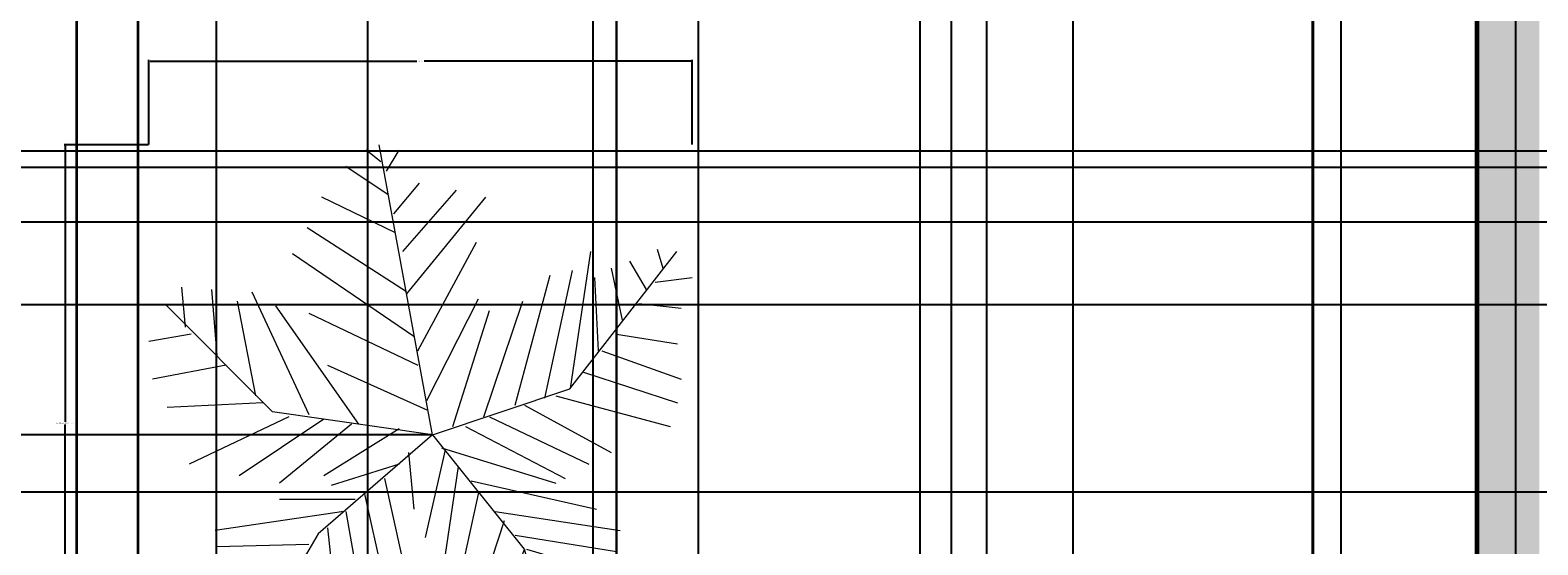
# Model space of a CAD drawing. Units: inches. Extents: x 818 to 1898, y 976 to 2364.
# Tile 8 of 96: x 986 to 1207, y 1592 to 1668. Entities that reach past the tile are written whole.
import ezdxf

# ---------------------------------------------------------------- set-up
doc = ezdxf.new("R2010")
doc.units = ezdxf.units.IN
doc.header["$LTSCALE"] = 5
doc.header["$MEASUREMENT"] = 0
for name, color, linetype, lineweight in [('A-ANNO-DIMS', 2, 'Continuous', 18), ('A-WALL', 7, 'Continuous', 40), ('C-PROP', 7, 'Continuous', 35), ('L-PLNT-BEDS', 94, 'Continuous', 18)]:
    doc.layers.add(name, color=color, linetype=linetype, lineweight=lineweight)
doc.layers.add('A-WALL-PATT', color=251, linetype='Continuous', lineweight=13, true_color=0x636466)
doc.layers.add('L-PLNT', color=116, linetype='Continuous', lineweight=13, true_color=0x136734)
doc.styles.get("Standard").update_dxf_attribs({"font": 'arial.ttf'})
doc.dimstyles.get("Standard").update_dxf_attribs({"dimtxt": 0.18, "dimasz": 0.18, "dimexe": 0.18, "dimexo": 0.0625, "dimgap": 0.09, "dimtad": 0, "dimtih": 1, "dimtoh": 1, "dimdec": 4, "dimzin": 0, "dimdsep": 46, "dimtxsty": 'Standard', "dimcen": 0.09, "dimadec": 0, "dimazin": 0, "dimtfac": 1, "dimtdec": 4, "dimtofl": 0, "dimtmove": 0, "dimatfit": 3, "dimfxl": 1, "dimtolj": 1, "dimtzin": 0, "dimarcsym": 0})

# ---------------------------------------------------------------- blocks, each defined once
blk = doc.blocks.new('PALM-BORDER')
for p, q in [((33.95, 78.95), (31.8, 80.68)), ((41.53, 39.05), (33.72, 81.45)), ((34.76, 77.57), (36.65, 80.68)), ((35.03, 74.11), (28.83, 78.26)), ((35.84, 71.35), (39.61, 75.84)), ((36.11, 68.59), (25.33, 73.77)), ((37.18, 65.82), (45, 74.8)), ((37.72, 59.6), (49.31, 73.77)), ((37.72, 59.95), (23.17, 69.28)), ((39.34, 51.31), (47.96, 67.2)), ((74.37, 66.17), (75.18, 63.4)), ((38.8, 53.39), (21.02, 65.48)), ((61.61, 45.75), (77.23, 65.83)), ((61.71, 45.79), (64.67, 65.82)), ((70.33, 64.44), (72.75, 60.3)), ((53.62, 43.37), (58.74, 62.37)), ((57.93, 44.41), (61.97, 63.06)), ((65.21, 62.02), (65.75, 51.31)), ((67.63, 63.4), (69.25, 55.81)), ((74.1, 61.33), (79.49, 62.02)), ((5.39, 54.77), (4.85, 60.64)), ((9.16, 60.3), (9.97, 50.62)), ((15.09, 59.95), (23.44, 41.99)), ((18.1, 42.4), (2.48, 58.02)), ((12.93, 58.57), (15.63, 44.75)), ((30.72, 40.61), (18.59, 57.88)), ((40.69, 44.06), (48.23, 58.91)), ((49.04, 41.64), (54.7, 58.57)), ((71.68, 58.22), (77.87, 57.53)), ((23.44, 56.84), (39.34, 49.24)), ((44.46, 40.26), (49.85, 57.19)), ((6.2, 53.73), (0, 52.7)), ((68.44, 53.73), (77.33, 52.35)), ((66.29, 51.31), (77.87, 47.17)), ((11.32, 49.24), (0.54, 47.17)), ((26.14, 49.24), (40.69, 42.68)), ((63.59, 48.21), (77.33, 43.71)), ((41.53, 39.05), (61.61, 45.75)), ((59.55, 44.75), (76.26, 40.26)), ((16.71, 43.71), (2.69, 43.02)), ((41.53, 39.05), (18.1, 42.4)), ((54.97, 43.37), (67.63, 36.46)), ((20.48, 41.64), (5.93, 34.73)), ((25.6, 41.3), (13.2, 33.01)), ((29.64, 40.61), (19.13, 31.97)), ((36.65, 39.91), (25.6, 33.01)), ((46.35, 40.26), (60.9, 32.66)), ((49.85, 41.64), (64.4, 34.73)), ((41.53, 39.05), (24.79, 24.55)), ((41.53, 39.05), (54.92, 22.32)), ((37.99, 36.46), (38.8, 28.17)), ((43.38, 36.81), (40.42, 24.02)), ((42.84, 37.15), (59.55, 31.97)), ((36.65, 34.73), (26.68, 31.62)), ((45.27, 34.39), (43.11, 19.88)), ((34.49, 32.66), (36.92, 21.61)), ((47.15, 32.32), (65.48, 28.17)), ((30.18, 29.55), (19.13, 29.55)), ((31.53, 30.59), (35.03, 14.7)), ((48.23, 30.59), (44.19, 12.28)), ((28.56, 27.82), (9.7, 25.06)), ((28.83, 27.82), (32.07, 9.17)), ((50.66, 27.82), (68.98, 25.06)), ((24.79, 24.55), (13.63, 5.58)), ((26.14, 25.41), (28.29, 6.06)), ((52, 26.44), (46.35, 9.17)), ((53.62, 24.37), (68.44, 21.95)), ((23.44, 22.99), (9.97, 22.64)), ((54.97, 22.3), (47.69, 5.02)), ((54.92, 22.32), (61.61, 0)), ((55.24, 22.3), (71.68, 17.46)), ((21.56, 19.53), (11.59, 19.88)), ((22.9, 21.26), (24.52, 5.37)), ((55.78, 20.22), (70.33, 14.35)), ((20.48, 17.46), (9.7, 15.73)), ((19.94, 16.08), (20.75, 6.41)), ((56.59, 16.42), (53.35, 5.72)), ((18.59, 13.66), (9.97, 12.62)), ((57.39, 14.7), (70.6, 8.83)), ((17.24, 11.59), (17.78, 6.06)), ((15.9, 9.52), (11.05, 7.44)), ((58.47, 10.9), (56.05, 2.95)), ((58.47, 10.55), (67.09, 5.72)), ((59.82, 6.75), (64.4, 3.64)), ((59.82, 5.02), (58.74, 1.22)), ((61.44, 1.92), (62.51, 1.22))]:
    blk.add_line(p, q)
blk = doc.blocks.new('*D26')
at = {"layer": 'A-ANNO-DIMS', "color": 0, "lineweight": -2, "ltscale": 5, "transparency": 16777216}
for p, q in [((1003.26, 1650.91), (990.92, 1650.91)), ((991.1, 1650.73), (991.1, 1610.37)), ((991.1, 1569.64), (991.1, 1610)), ((1003.26, 1569.46), (990.92, 1569.46))]:
    blk.add_line(p, q, dxfattribs=at)
at = {"layer": 'A-ANNO-DIMS', "color": 0, "ltscale": 5, "transparency": 16777216}
for points in [[(991.07, 1650.73), (991.13, 1650.73), (991.1, 1650.91)], [(991.07, 1569.64), (991.13, 1569.64), (991.1, 1569.46)]]:
    blk.add_solid(points, dxfattribs=at)
at = {"layer": 'Defpoints', "color": 0, "ltscale": 5, "transparency": 16777216}
for p in [(991.1, 1650.91), (1003.32, 1650.91), (1003.32, 1569.46)]:
    blk.add_point(p, dxfattribs=at)
at = {"layer": 'A-ANNO-DIMS', "color": 0, "ltscale": 5, "transparency": 16777216, "insert": (991.1, 1610.19), "char_height": 0.18, "attachment_point": 5}
blk.add_mtext('\\A1;BORDER PALM 81 TYP.', dxfattribs=at)
blk = doc.blocks.new('*D27')
at = {"layer": 'A-ANNO-DIMS', "color": 0, "lineweight": -2, "ltscale": 5, "transparency": 16777216}
for p, q in [((1003.32, 1650.97), (1003.32, 1663.31)), ((1003.5, 1663.13), (1042.54, 1663.13)), ((1082.63, 1663.13), (1043.59, 1663.13)), ((1082.81, 1650.97), (1082.81, 1663.31))]:
    blk.add_line(p, q, dxfattribs=at)
at = {"layer": 'A-ANNO-DIMS', "color": 0, "ltscale": 5, "transparency": 16777216}
for points in [[(1003.5, 1663.16), (1003.5, 1663.1), (1003.32, 1663.13)], [(1082.63, 1663.16), (1082.63, 1663.1), (1082.81, 1663.13)]]:
    blk.add_solid(points, dxfattribs=at)
at = {"layer": 'Defpoints', "color": 0, "ltscale": 5, "transparency": 16777216}
for p in [(1082.81, 1663.13), (1003.32, 1650.91), (1082.81, 1650.91)]:
    blk.add_point(p, dxfattribs=at)
at = {"layer": 'A-ANNO-DIMS', "color": 0, "ltscale": 5, "transparency": 16777216, "insert": (1043.06, 1663.13), "char_height": 0.18, "attachment_point": 5}
blk.add_mtext('\\A1;79 TYP.', dxfattribs=at)
blk = doc.blocks.new('*D59')
at = {"layer": 'A-ANNO-DIMS', "color": 0, "lineweight": -2, "ltscale": 5, "transparency": 16777216}
for p, q in [((1251.64, 2300.39), (818.03, 2300.39)), ((818.21, 2300.21), (818.21, 1669.95)), ((818.21, 1039.32), (818.21, 1669.59)), ((896.05, 1039.14), (818.03, 1039.14))]:
    blk.add_line(p, q, dxfattribs=at)
at = {"layer": 'A-ANNO-DIMS', "color": 0, "ltscale": 5, "transparency": 16777216}
for points in [[(818.18, 2300.21), (818.24, 2300.21), (818.21, 2300.39)], [(818.18, 1039.32), (818.24, 1039.32), (818.21, 1039.14)]]:
    blk.add_solid(points, dxfattribs=at)
at = {"layer": 'Defpoints', "color": 0, "ltscale": 5, "transparency": 16777216}
for p in [(818.21, 2300.39), (1251.71, 2300.39), (896.11, 1039.14)]:
    blk.add_point(p, dxfattribs=at)
at = {"layer": 'A-ANNO-DIMS', "color": 0, "ltscale": 5, "transparency": 16777216, "insert": (818.21, 1669.77), "char_height": 0.18, "attachment_point": 5}
blk.add_mtext('\\A1;1261.2', dxfattribs=at)
blk = doc.blocks.new('*D60')
at = {"layer": 'A-ANNO-DIMS', "color": 0, "lineweight": -2, "ltscale": 5, "transparency": 16777216}
for p, q in [((992.66, 2294.22), (818.03, 2294.22)), ((818.21, 2294.04), (818.21, 1748.77)), ((818.21, 1203.14), (818.21, 1748.41)), ((992.66, 1202.96), (818.03, 1202.96))]:
    blk.add_line(p, q, dxfattribs=at)
at = {"layer": 'A-ANNO-DIMS', "color": 0, "ltscale": 5, "transparency": 16777216}
for points in [[(818.18, 2294.04), (818.24, 2294.04), (818.21, 2294.22)], [(818.18, 1203.14), (818.24, 1203.14), (818.21, 1202.96)]]:
    blk.add_solid(points, dxfattribs=at)
at = {"layer": 'Defpoints', "color": 0, "ltscale": 5, "transparency": 16777216}
for p in [(818.21, 2294.22), (992.73, 2294.22), (992.73, 1202.96)]:
    blk.add_point(p, dxfattribs=at)
at = {"layer": 'A-ANNO-DIMS', "color": 0, "ltscale": 5, "transparency": 16777216, "insert": (818.21, 1748.59), "char_height": 0.18, "attachment_point": 5}
blk.add_mtext('\\A1;1091.3', dxfattribs=at)
blk = doc.blocks.new('*D61')
at = {"layer": 'A-ANNO-DIMS', "color": 0, "lineweight": -2, "ltscale": 5, "transparency": 16777216}
for p, q in [((1071.73, 1203.03), (1071.73, 2363.87)), ((1071.91, 2363.69), (1250.94, 2363.69)), ((1430.55, 2363.69), (1251.51, 2363.69)), ((1430.73, 1203.03), (1430.73, 2363.87))]:
    blk.add_line(p, q, dxfattribs=at)
at = {"layer": 'A-ANNO-DIMS', "color": 0, "ltscale": 5, "transparency": 16777216}
for points in [[(1071.91, 2363.72), (1071.91, 2363.66), (1071.73, 2363.69)], [(1430.55, 2363.72), (1430.55, 2363.66), (1430.73, 2363.69)]]:
    blk.add_solid(points, dxfattribs=at)
at = {"layer": 'Defpoints', "color": 0, "ltscale": 5, "transparency": 16777216}
for p in [(1430.73, 2363.69), (1071.73, 1202.96), (1430.73, 1202.96)]:
    blk.add_point(p, dxfattribs=at)
at = {"layer": 'A-ANNO-DIMS', "color": 0, "ltscale": 5, "transparency": 16777216, "insert": (1251.23, 2363.69), "char_height": 0.18, "attachment_point": 5}
blk.add_mtext('\\A1;359', dxfattribs=at)
blk = doc.blocks.new('*D64')
at = {"layer": 'A-ANNO-DIMS', "color": 0, "lineweight": -2, "ltscale": 5, "transparency": 16777216}
for p, q in [((1197.73, 1501.14), (1197.73, 2363.87)), ((1197.91, 2363.69), (1313.93, 2363.69)), ((1430.55, 2363.69), (1314.52, 2363.69)), ((1430.73, 1501.14), (1430.73, 2363.87))]:
    blk.add_line(p, q, dxfattribs=at)
at = {"layer": 'A-ANNO-DIMS', "color": 0, "ltscale": 5, "transparency": 16777216}
for points in [[(1197.91, 2363.72), (1197.91, 2363.66), (1197.73, 2363.69)], [(1430.55, 2363.72), (1430.55, 2363.66), (1430.73, 2363.69)]]:
    blk.add_solid(points, dxfattribs=at)
at = {"layer": 'Defpoints', "color": 0, "ltscale": 5, "transparency": 16777216}
for p in [(1430.73, 2363.69), (1197.73, 1501.08), (1430.73, 1501.08)]:
    blk.add_point(p, dxfattribs=at)
at = {"layer": 'A-ANNO-DIMS', "color": 0, "ltscale": 5, "transparency": 16777216, "insert": (1314.23, 2363.69), "char_height": 0.18, "attachment_point": 5}
blk.add_mtext('\\A1;233', dxfattribs=at)
blk = doc.blocks.new('*D79')
at = {"layer": 'A-ANNO-DIMS', "color": 0, "lineweight": -2, "ltscale": 5, "transparency": 16777216}
for p, q in [((992.73, 1203.03), (992.73, 2363.87)), ((992.91, 2363.69), (1032.01, 2363.69)), ((1071.55, 2363.69), (1032.44, 2363.69)), ((1071.73, 1203.03), (1071.73, 2363.87))]:
    blk.add_line(p, q, dxfattribs=at)
at = {"layer": 'A-ANNO-DIMS', "color": 0, "ltscale": 5, "transparency": 16777216}
for points in [[(992.91, 2363.72), (992.91, 2363.66), (992.73, 2363.69)], [(1071.55, 2363.72), (1071.55, 2363.66), (1071.73, 2363.69)]]:
    blk.add_solid(points, dxfattribs=at)
at = {"layer": 'Defpoints', "color": 0, "ltscale": 5, "transparency": 16777216}
for p in [(1071.73, 2363.69), (992.73, 1202.96), (1071.73, 1202.96)]:
    blk.add_point(p, dxfattribs=at)
at = {"layer": 'A-ANNO-DIMS', "color": 0, "ltscale": 5, "transparency": 16777216, "insert": (1032.23, 2363.69), "char_height": 0.18, "attachment_point": 5}
blk.add_mtext('\\A1;79', dxfattribs=at)
blk = doc.blocks.new('*D82')
at = {"layer": 'A-ANNO-DIMS', "color": 0, "lineweight": -2, "ltscale": 5, "transparency": 16777216}
for p, q in [((1083.73, 1501.14), (1083.73, 2363.87)), ((1083.91, 2363.69), (1140.45, 2363.69)), ((1197.55, 2363.69), (1141.01, 2363.69)), ((1197.73, 1501.14), (1197.73, 2363.87))]:
    blk.add_line(p, q, dxfattribs=at)
at = {"layer": 'A-ANNO-DIMS', "color": 0, "ltscale": 5, "transparency": 16777216}
for points in [[(1083.91, 2363.72), (1083.91, 2363.66), (1083.73, 2363.69)], [(1197.55, 2363.72), (1197.55, 2363.66), (1197.73, 2363.69)]]:
    blk.add_solid(points, dxfattribs=at)
at = {"layer": 'Defpoints', "color": 0, "ltscale": 5, "transparency": 16777216}
for p in [(1197.73, 2363.69), (1083.73, 1501.08), (1197.73, 1501.08)]:
    blk.add_point(p, dxfattribs=at)
at = {"layer": 'A-ANNO-DIMS', "color": 0, "ltscale": 5, "transparency": 16777216, "insert": (1140.73, 2363.69), "char_height": 0.18, "attachment_point": 5}
blk.add_mtext('\\A1;114', dxfattribs=at)
blk = doc.blocks.new('*D84')
at = {"layer": 'A-ANNO-DIMS', "color": 0, "lineweight": -2, "ltscale": 5, "transparency": 16777216}
for p, q in [((1197.66, 1700.08), (818.03, 1700.08)), ((818.21, 1699.9), (818.21, 1600.76)), ((818.21, 1501.26), (818.21, 1600.4)), ((1197.66, 1501.08), (818.03, 1501.08))]:
    blk.add_line(p, q, dxfattribs=at)
at = {"layer": 'A-ANNO-DIMS', "color": 0, "ltscale": 5, "transparency": 16777216}
for points in [[(818.18, 1699.9), (818.24, 1699.9), (818.21, 1700.08)], [(818.18, 1501.26), (818.24, 1501.26), (818.21, 1501.08)]]:
    blk.add_solid(points, dxfattribs=at)
at = {"layer": 'Defpoints', "color": 0, "ltscale": 5, "transparency": 16777216}
for p in [(818.21, 1700.08), (1197.73, 1700.08), (1197.73, 1501.08)]:
    blk.add_point(p, dxfattribs=at)
at = {"layer": 'A-ANNO-DIMS', "color": 0, "ltscale": 5, "transparency": 16777216, "insert": (818.21, 1600.58), "char_height": 0.18, "attachment_point": 5}
blk.add_mtext('\\A1;199', dxfattribs=at)
blk = doc.blocks.new('*D91')
at = {"layer": 'A-ANNO-DIMS', "color": 0, "lineweight": -2, "ltscale": 5, "transparency": 16777216}
for p, q in [((959.17, 1071.12), (959.17, 2363.87)), ((959.35, 2363.69), (985.8, 2363.69)), ((1013.04, 2363.69), (986.59, 2363.69)), ((1013.22, 1071.12), (1013.22, 2363.87))]:
    blk.add_line(p, q, dxfattribs=at)
at = {"layer": 'A-ANNO-DIMS', "color": 0, "ltscale": 5, "transparency": 16777216}
for points in [[(959.35, 2363.72), (959.35, 2363.66), (959.17, 2363.69)], [(1013.04, 2363.72), (1013.04, 2363.66), (1013.22, 2363.69)]]:
    blk.add_solid(points, dxfattribs=at)
at = {"layer": 'Defpoints', "color": 0, "ltscale": 5, "transparency": 16777216}
for p in [(1013.22, 2363.69), (959.17, 1071.06), (1013.22, 1071.06)]:
    blk.add_point(p, dxfattribs=at)
at = {"layer": 'A-ANNO-DIMS', "color": 0, "ltscale": 5, "transparency": 16777216, "insert": (986.2, 2363.69), "char_height": 0.18, "attachment_point": 5}
blk.add_mtext('\\A1;54.04', dxfattribs=at)
blk = doc.blocks.new('*D92')
at = {"layer": 'A-ANNO-DIMS', "color": 0, "lineweight": -2, "ltscale": 5, "transparency": 16777216}
for p, q in [((1013.22, 1071.12), (1013.22, 2363.87)), ((1013.4, 2363.69), (1040.38, 2363.69)), ((1068.16, 2363.69), (1041.17, 2363.69)), ((1068.34, 1071.12), (1068.34, 2363.87))]:
    blk.add_line(p, q, dxfattribs=at)
at = {"layer": 'A-ANNO-DIMS', "color": 0, "ltscale": 5, "transparency": 16777216}
for points in [[(1013.4, 2363.72), (1013.4, 2363.66), (1013.22, 2363.69)], [(1068.16, 2363.72), (1068.16, 2363.66), (1068.34, 2363.69)]]:
    blk.add_solid(points, dxfattribs=at)
at = {"layer": 'Defpoints', "color": 0, "ltscale": 5, "transparency": 16777216}
for p in [(1068.34, 2363.69), (1013.22, 1071.06), (1068.34, 1071.06)]:
    blk.add_point(p, dxfattribs=at)
at = {"layer": 'A-ANNO-DIMS', "color": 0, "ltscale": 5, "transparency": 16777216, "insert": (1040.78, 2363.69), "char_height": 0.18, "attachment_point": 5}
blk.add_mtext('\\A1;55.12', dxfattribs=at)
blk = doc.blocks.new('*D93')
at = {"layer": 'A-ANNO-DIMS', "color": 0, "lineweight": -2, "ltscale": 5, "transparency": 16777216}
for p, q in [((1068.34, 1071.12), (1068.34, 2363.87)), ((1068.52, 2363.69), (1094.16, 2363.69)), ((1120.58, 2363.69), (1094.94, 2363.69)), ((1120.76, 1071.12), (1120.76, 2363.87))]:
    blk.add_line(p, q, dxfattribs=at)
at = {"layer": 'A-ANNO-DIMS', "color": 0, "ltscale": 5, "transparency": 16777216}
for points in [[(1068.52, 2363.72), (1068.52, 2363.66), (1068.34, 2363.69)], [(1120.58, 2363.72), (1120.58, 2363.66), (1120.76, 2363.69)]]:
    blk.add_solid(points, dxfattribs=at)
at = {"layer": 'Defpoints', "color": 0, "ltscale": 5, "transparency": 16777216}
for p in [(1120.76, 2363.69), (1068.34, 1071.06), (1120.76, 1071.06)]:
    blk.add_point(p, dxfattribs=at)
at = {"layer": 'A-ANNO-DIMS', "color": 0, "ltscale": 5, "transparency": 16777216, "insert": (1094.55, 2363.69), "char_height": 0.18, "attachment_point": 5}
blk.add_mtext('\\A1;52.42', dxfattribs=at)
blk = doc.blocks.new('*D94')
at = {"layer": 'A-ANNO-DIMS', "color": 0, "lineweight": -2, "ltscale": 5, "transparency": 16777216}
for p, q in [((1120.76, 1071.12), (1120.76, 2363.87)), ((1120.94, 2363.69), (1146.76, 2363.69)), ((1173.36, 2363.69), (1147.55, 2363.69)), ((1173.54, 1071.12), (1173.54, 2363.87))]:
    blk.add_line(p, q, dxfattribs=at)
at = {"layer": 'A-ANNO-DIMS', "color": 0, "ltscale": 5, "transparency": 16777216}
for points in [[(1120.94, 2363.72), (1120.94, 2363.66), (1120.76, 2363.69)], [(1173.36, 2363.72), (1173.36, 2363.66), (1173.54, 2363.69)]]:
    blk.add_solid(points, dxfattribs=at)
at = {"layer": 'Defpoints', "color": 0, "ltscale": 5, "transparency": 16777216}
for p in [(1173.54, 2363.69), (1120.76, 1071.06), (1173.54, 1071.06)]:
    blk.add_point(p, dxfattribs=at)
at = {"layer": 'A-ANNO-DIMS', "color": 0, "ltscale": 5, "transparency": 16777216, "insert": (1147.15, 2363.69), "char_height": 0.18, "attachment_point": 5}
blk.add_mtext('\\A1;52.78', dxfattribs=at)
blk = doc.blocks.new('*D95')
at = {"layer": 'A-ANNO-DIMS', "color": 0, "lineweight": -2, "ltscale": 5, "transparency": 16777216}
for p, q in [((1173.54, 1071.12), (1173.54, 2363.87)), ((1173.72, 2363.69), (1201.29, 2363.69)), ((1229.47, 2363.69), (1201.9, 2363.69)), ((1229.65, 1071.12), (1229.65, 2363.87))]:
    blk.add_line(p, q, dxfattribs=at)
at = {"layer": 'A-ANNO-DIMS', "color": 0, "ltscale": 5, "transparency": 16777216}
for points in [[(1173.72, 2363.72), (1173.72, 2363.66), (1173.54, 2363.69)], [(1229.47, 2363.72), (1229.47, 2363.66), (1229.65, 2363.69)]]:
    blk.add_solid(points, dxfattribs=at)
at = {"layer": 'Defpoints', "color": 0, "ltscale": 5, "transparency": 16777216}
for p in [(1229.65, 2363.69), (1173.54, 1071.06), (1229.65, 1071.06)]:
    blk.add_point(p, dxfattribs=at)
at = {"layer": 'A-ANNO-DIMS', "color": 0, "ltscale": 5, "transparency": 16777216, "insert": (1201.59, 2363.69), "char_height": 0.18, "attachment_point": 5}
blk.add_mtext('\\A1;56.1', dxfattribs=at)
blk = doc.blocks.new('*D109')
at = {"layer": 'A-ANNO-DIMS', "color": 0, "lineweight": -2, "ltscale": 5, "transparency": 16777216}
for p, q in [((1125.92, 1410.12), (1125.92, 2363.87)), ((1126.1, 2363.69), (1164.25, 2363.69)), ((1203.15, 2363.69), (1165, 2363.69)), ((1203.33, 1409.91), (1203.33, 2363.87))]:
    blk.add_line(p, q, dxfattribs=at)
at = {"layer": 'A-ANNO-DIMS', "color": 0, "ltscale": 5, "transparency": 16777216}
for points in [[(1126.1, 2363.72), (1126.1, 2363.66), (1125.92, 2363.69)], [(1203.15, 2363.72), (1203.15, 2363.66), (1203.33, 2363.69)]]:
    blk.add_solid(points, dxfattribs=at)
at = {"layer": 'Defpoints', "color": 0, "ltscale": 5, "transparency": 16777216}
for p in [(1203.33, 2363.69), (1125.92, 1410.05), (1203.33, 1409.85)]:
    blk.add_point(p, dxfattribs=at)
at = {"layer": 'A-ANNO-DIMS', "color": 0, "ltscale": 5, "transparency": 16777216, "insert": (1164.62, 2363.69), "char_height": 0.18, "attachment_point": 5}
blk.add_mtext('\\A1;77.41', dxfattribs=at)
blk = doc.blocks.new('*D118')
at = {"layer": 'A-ANNO-DIMS', "color": 0, "lineweight": -2, "ltscale": 5, "transparency": 16777216}
for p, q in [((1766.29, 1627.51), (818.03, 1627.51)), ((818.21, 1627.33), (818.21, 1586.53)), ((818.21, 1545.36), (818.21, 1586.16)), ((1766.29, 1545.18), (818.03, 1545.18))]:
    blk.add_line(p, q, dxfattribs=at)
at = {"layer": 'A-ANNO-DIMS', "color": 0, "ltscale": 5, "transparency": 16777216}
for points in [[(818.18, 1627.33), (818.24, 1627.33), (818.21, 1627.51)], [(818.18, 1545.36), (818.24, 1545.36), (818.21, 1545.18)]]:
    blk.add_solid(points, dxfattribs=at)
at = {"layer": 'Defpoints', "color": 0, "ltscale": 5, "transparency": 16777216}
for p in [(818.21, 1627.51), (1766.35, 1627.51), (1766.35, 1545.18)]:
    blk.add_point(p, dxfattribs=at)
at = {"layer": 'A-ANNO-DIMS', "color": 0, "ltscale": 5, "transparency": 16777216, "insert": (818.21, 1586.34), "char_height": 0.18, "attachment_point": 5}
blk.add_mtext('\\A1;82.32', dxfattribs=at)
blk = doc.blocks.new('*D119')
at = {"layer": 'A-ANNO-DIMS', "color": 0, "lineweight": -2, "ltscale": 5, "transparency": 16777216}
for p, q in [((1766.29, 1716.99), (818.03, 1716.99)), ((818.21, 1716.81), (818.21, 1672.43)), ((818.21, 1627.69), (818.21, 1672.06)), ((1766.29, 1627.51), (818.03, 1627.51))]:
    blk.add_line(p, q, dxfattribs=at)
at = {"layer": 'A-ANNO-DIMS', "color": 0, "ltscale": 5, "transparency": 16777216}
for points in [[(818.18, 1716.81), (818.24, 1716.81), (818.21, 1716.99)], [(818.18, 1627.69), (818.24, 1627.69), (818.21, 1627.51)]]:
    blk.add_solid(points, dxfattribs=at)
at = {"layer": 'Defpoints', "color": 0, "ltscale": 5, "transparency": 16777216}
for p in [(818.21, 1716.99), (1766.35, 1716.99), (1766.35, 1627.51)]:
    blk.add_point(p, dxfattribs=at)
at = {"layer": 'A-ANNO-DIMS', "color": 0, "ltscale": 5, "transparency": 16777216, "insert": (818.21, 1672.25), "char_height": 0.18, "attachment_point": 5}
blk.add_mtext('\\A1;89.48', dxfattribs=at)
blk = doc.blocks.new('*D122')
at = {"layer": 'A-ANNO-DIMS', "color": 0, "lineweight": -2, "ltscale": 5, "transparency": 16777216}
for p, q in [((1138.5, 1794.37), (1138.5, 975.66)), ((1071.73, 1688.02), (1071.73, 975.66)), ((1071.91, 975.84), (1104.72, 975.84)), ((1138.32, 975.84), (1105.51, 975.84))]:
    blk.add_line(p, q, dxfattribs=at)
at = {"layer": 'A-ANNO-DIMS', "color": 0, "ltscale": 5, "transparency": 16777216}
for points in [[(1071.91, 975.87), (1071.91, 975.81), (1071.73, 975.84)], [(1138.32, 975.87), (1138.32, 975.81), (1138.5, 975.84)]]:
    blk.add_solid(points, dxfattribs=at)
at = {"layer": 'Defpoints', "color": 0, "ltscale": 5, "transparency": 16777216}
for p in [(1138.5, 1794.43), (1071.73, 1688.08), (1138.5, 975.84)]:
    blk.add_point(p, dxfattribs=at)
at = {"layer": 'A-ANNO-DIMS', "color": 0, "ltscale": 5, "transparency": 16777216, "insert": (1105.11, 975.84), "char_height": 0.18, "attachment_point": 5}
blk.add_mtext('\\A1;66.78', dxfattribs=at)
blk = doc.blocks.new('*D126')
at = {"layer": 'A-ANNO-DIMS', "color": 0, "lineweight": -2, "ltscale": 5, "transparency": 16777216}
for p, q in [((1035.38, 1252.09), (1035.38, 2363.87)), ((1035.56, 2363.69), (1075.41, 2363.69)), ((1116.01, 2363.69), (1076.16, 2363.69)), ((1116.19, 1236.03), (1116.19, 2363.87))]:
    blk.add_line(p, q, dxfattribs=at)
at = {"layer": 'A-ANNO-DIMS', "color": 0, "ltscale": 5, "transparency": 16777216}
for points in [[(1035.56, 2363.72), (1035.56, 2363.66), (1035.38, 2363.69)], [(1116.01, 2363.72), (1116.01, 2363.66), (1116.19, 2363.69)]]:
    blk.add_solid(points, dxfattribs=at)
at = {"layer": 'Defpoints', "color": 0, "ltscale": 5, "transparency": 16777216}
for p in [(1035.38, 2363.69), (1035.38, 1252.02), (1116.19, 1235.96)]:
    blk.add_point(p, dxfattribs=at)
at = {"layer": 'A-ANNO-DIMS', "color": 0, "ltscale": 5, "transparency": 16777216, "insert": (1075.78, 2363.69), "char_height": 0.18, "attachment_point": 5}
blk.add_mtext('\\A1;80.81', dxfattribs=at)
blk = doc.blocks.new('*D129')
at = {"layer": 'A-ANNO-DIMS', "color": 0, "lineweight": -2, "ltscale": 5, "transparency": 16777216}
for p, q in [((1044.78, 1608.51), (818.03, 1608.51)), ((818.21, 1608.33), (818.21, 1521.27)), ((818.21, 1433.85), (818.21, 1520.91)), ((1044.78, 1433.67), (818.03, 1433.67))]:
    blk.add_line(p, q, dxfattribs=at)
at = {"layer": 'A-ANNO-DIMS', "color": 0, "ltscale": 5, "transparency": 16777216}
for points in [[(818.18, 1608.33), (818.24, 1608.33), (818.21, 1608.51)], [(818.18, 1433.85), (818.24, 1433.85), (818.21, 1433.67)]]:
    blk.add_solid(points, dxfattribs=at)
at = {"layer": 'Defpoints', "color": 0, "ltscale": 5, "transparency": 16777216}
for p in [(818.21, 1608.51), (1044.85, 1608.51), (1044.85, 1433.67)]:
    blk.add_point(p, dxfattribs=at)
at = {"layer": 'A-ANNO-DIMS', "color": 0, "ltscale": 5, "transparency": 16777216, "insert": (818.21, 1521.09), "char_height": 0.18, "attachment_point": 5}
blk.add_mtext('\\A1;174.84', dxfattribs=at)
blk = doc.blocks.new('*D130')
at = {"layer": 'A-ANNO-DIMS', "color": 0, "lineweight": -2, "ltscale": 5, "transparency": 16777216}
for p, q in [((1044.78, 1724.63), (818.03, 1724.63)), ((818.21, 1724.45), (818.21, 1666.75)), ((818.21, 1608.69), (818.21, 1666.39)), ((1044.78, 1608.51), (818.03, 1608.51))]:
    blk.add_line(p, q, dxfattribs=at)
at = {"layer": 'A-ANNO-DIMS', "color": 0, "ltscale": 5, "transparency": 16777216}
for points in [[(818.18, 1724.45), (818.24, 1724.45), (818.21, 1724.63)], [(818.18, 1608.69), (818.24, 1608.69), (818.21, 1608.51)]]:
    blk.add_solid(points, dxfattribs=at)
at = {"layer": 'Defpoints', "color": 0, "ltscale": 5, "transparency": 16777216}
for p in [(818.21, 1724.63), (1044.85, 1724.63), (1044.85, 1608.51)]:
    blk.add_point(p, dxfattribs=at)
at = {"layer": 'A-ANNO-DIMS', "color": 0, "ltscale": 5, "transparency": 16777216, "insert": (818.21, 1666.57), "char_height": 0.18, "attachment_point": 5}
blk.add_mtext('\\A1;116.12', dxfattribs=at)
blk = doc.blocks.new('*D145')
at = {"layer": 'A-ANNO-DIMS', "color": 0, "lineweight": -2, "ltscale": 5, "transparency": 16777216}
for p, q in [((1197.39, 2122.31), (1197.39, 975.66)), ((1232.61, 2122.31), (1232.61, 975.66)), ((1197.57, 975.84), (1214.61, 975.84)), ((1232.43, 975.84), (1215.39, 975.84))]:
    blk.add_line(p, q, dxfattribs=at)
at = {"layer": 'A-ANNO-DIMS', "color": 0, "ltscale": 5, "transparency": 16777216}
for points in [[(1197.57, 975.87), (1197.57, 975.81), (1197.39, 975.84)], [(1232.43, 975.87), (1232.43, 975.81), (1232.61, 975.84)]]:
    blk.add_solid(points, dxfattribs=at)
at = {"layer": 'Defpoints', "color": 0, "ltscale": 5, "transparency": 16777216}
for p in [(1197.39, 2122.38), (1232.61, 2122.38), (1232.61, 975.84)]:
    blk.add_point(p, dxfattribs=at)
at = {"layer": 'A-ANNO-DIMS', "color": 0, "ltscale": 5, "transparency": 16777216, "insert": (1215, 975.84), "char_height": 0.18, "attachment_point": 5}
blk.add_mtext('\\A1;35.22', dxfattribs=at)
blk = doc.blocks.new('*D158')
at = {"layer": 'A-ANNO-DIMS', "color": 0, "lineweight": -2, "ltscale": 5, "transparency": 16777216}
for p, q in [((1173.73, 1590.82), (1173.73, 2363.87)), ((1173.91, 2363.69), (1175.57, 2363.69)), ((1177.55, 2363.69), (1175.88, 2363.69)), ((1177.73, 1586.82), (1177.73, 2363.87))]:
    blk.add_line(p, q, dxfattribs=at)
at = {"layer": 'A-ANNO-DIMS', "color": 0, "ltscale": 5, "transparency": 16777216}
for points in [[(1173.91, 2363.72), (1173.91, 2363.66), (1173.73, 2363.69)], [(1177.55, 2363.72), (1177.55, 2363.66), (1177.73, 2363.69)]]:
    blk.add_solid(points, dxfattribs=at)
at = {"layer": 'Defpoints', "color": 0, "ltscale": 5, "transparency": 16777216}
for p in [(1177.73, 2363.69), (1173.73, 1590.76), (1177.73, 1586.76)]:
    blk.add_point(p, dxfattribs=at)
at = {"layer": 'A-ANNO-DIMS', "color": 0, "ltscale": 5, "transparency": 16777216, "insert": (1175.73, 2363.69), "char_height": 0.18, "attachment_point": 5}
blk.add_mtext('\\A1;4', dxfattribs=at)
blk = doc.blocks.new('*D176')
at = {"layer": 'A-ANNO-DIMS', "color": 0, "lineweight": -2, "ltscale": 5, "transparency": 16777216}
for p, q in [((1559.66, 1687.08), (818.03, 1687.08)), ((818.21, 1686.9), (818.21, 1667.51)), ((818.21, 1647.76), (818.21, 1667.15)), ((1559.66, 1647.58), (818.03, 1647.58))]:
    blk.add_line(p, q, dxfattribs=at)
at = {"layer": 'A-ANNO-DIMS', "color": 0, "ltscale": 5, "transparency": 16777216}
for points in [[(818.18, 1686.9), (818.24, 1686.9), (818.21, 1687.08)], [(818.18, 1647.76), (818.24, 1647.76), (818.21, 1647.58)]]:
    blk.add_solid(points, dxfattribs=at)
at = {"layer": 'Defpoints', "color": 0, "ltscale": 5, "transparency": 16777216}
for p in [(1559.73, 1687.08), (818.21, 1647.58), (1559.73, 1647.58)]:
    blk.add_point(p, dxfattribs=at)
at = {"layer": 'A-ANNO-DIMS', "color": 0, "ltscale": 5, "transparency": 16777216, "insert": (818.21, 1667.33), "char_height": 0.18, "attachment_point": 5}
blk.add_mtext('\\A1;39.5', dxfattribs=at)
blk = doc.blocks.new('*D181')
at = {"layer": 'A-ANNO-DIMS', "color": 0, "lineweight": -2, "ltscale": 5, "transparency": 16777216}
for p, q in [((1599.66, 1639.58), (818.03, 1639.58)), ((818.21, 1639.4), (818.21, 1620.01)), ((818.21, 1600.26), (818.21, 1619.65)), ((1619.66, 1600.08), (818.03, 1600.08))]:
    blk.add_line(p, q, dxfattribs=at)
at = {"layer": 'A-ANNO-DIMS', "color": 0, "ltscale": 5, "transparency": 16777216}
for points in [[(818.18, 1639.4), (818.24, 1639.4), (818.21, 1639.58)], [(818.18, 1600.26), (818.24, 1600.26), (818.21, 1600.08)]]:
    blk.add_solid(points, dxfattribs=at)
at = {"layer": 'Defpoints', "color": 0, "ltscale": 5, "transparency": 16777216}
for p in [(1599.73, 1639.58), (818.21, 1600.08), (1619.73, 1600.08)]:
    blk.add_point(p, dxfattribs=at)
at = {"layer": 'A-ANNO-DIMS', "color": 0, "ltscale": 5, "transparency": 16777216, "insert": (818.21, 1619.83), "char_height": 0.18, "attachment_point": 5}
blk.add_mtext('\\A1;39.5', dxfattribs=at)
blk = doc.blocks.new('*D277')
at = {"layer": 'A-ANNO-DIMS', "color": 0, "lineweight": -2, "ltscale": 5, "transparency": 16777216}
for p, q in [((1251.87, 1687.08), (818.03, 1687.08)), ((818.21, 1686.9), (818.21, 1668.7)), ((818.21, 1650.13), (818.21, 1668.33)), ((1256.59, 1649.95), (818.03, 1649.95))]:
    blk.add_line(p, q, dxfattribs=at)
at = {"layer": 'A-ANNO-DIMS', "color": 0, "ltscale": 5, "transparency": 16777216}
for points in [[(818.18, 1686.9), (818.24, 1686.9), (818.21, 1687.08)], [(818.18, 1650.13), (818.24, 1650.13), (818.21, 1649.95)]]:
    blk.add_solid(points, dxfattribs=at)
at = {"layer": 'Defpoints', "color": 0, "ltscale": 5, "transparency": 16777216}
for p in [(818.21, 1687.08), (1251.93, 1687.08), (1256.65, 1649.95)]:
    blk.add_point(p, dxfattribs=at)
at = {"layer": 'A-ANNO-DIMS', "color": 0, "ltscale": 5, "transparency": 16777216, "insert": (818.21, 1668.52), "char_height": 0.18, "attachment_point": 5}
blk.add_mtext('\\A1;37.13', dxfattribs=at)

msp = doc.modelspace()

# ---------------------------------------------------------------- hatches: boundary and pattern name
at = {"layer": 'A-WALL-PATT', "ltscale": 5}
h = msp.add_hatch(color=256, dxfattribs=at)
h.dxf.hatch_style = 1
h.paths.add_polyline_path([(1206.7252, 1687.0782), (1206.7252, 1700.0782), (1197.7251, 1700.0782), (1197.7251, 1501.0782), (1206.7252, 1501.0782), (1206.7252, 1510.0782)])
h.paths.add_polyline_path([(1197.7251, 1590.7585), (1173.7251, 1590.7585), (1173.7251, 1586.7585), (1197.7251, 1586.7585)])
h.paths.add_polyline_path([(1197.7251, 1534.6024), (1173.7251, 1534.6024), (1173.7251, 1530.6024), (1197.7251, 1530.6024)])
h.paths.add_polyline_path([(1365.1463, 1510.0782), (1283.8183, 1510.0782), (1283.8183, 1501.0782), (1365.1463, 1501.0782)])
h.paths.add_polyline_path([(1439.7252, 1591.0782), (1441.7252, 1591.0782), (1441.7252, 1600.0782), (1430.7251, 1600.0782), (1430.7251, 1510.0782), (1406.7252, 1510.0782), (1401.1463, 1510.0782), (1401.1463, 1501.0782), (1430.7251, 1501.0782), (1430.7251, 1486.2383), (1430.7251, 1409.0522), (1439.7252, 1409.0522)])

# ---------------------------------------------------------------- linework, layer by layer
at = {"layer": 'A-WALL'}
msp.add_line((1197.7251, 1700.0782), (1197.7251, 1501.0782), dxfattribs=at)
at = {"layer": 'C-PROP'}
for p, q in [((992.7251, 2294.2171), (992.7251, 1202.9642)), ((1001.7252, 2285.2171), (1001.7252, 1211.9642))]:
    msp.add_line(p, q, dxfattribs=at)
at = {"layer": 'L-PLNT-BEDS'}
for p, q in [((1071.7251, 2214.9709), (1071.7251, 1202.9642)), ((1083.7251, 2044.0782), (1083.7251, 1211.9642))]:
    msp.add_line(p, q, dxfattribs=at)

# ---------------------------------------------------------------- block references
at = {"layer": 'L-PLNT'}
msp.add_blockref('PALM-BORDER', (1003.3185, 1569.4605), dxfattribs=at)

# ---------------------------------------------------------------- dimensions: what is measured, and where the dimension line sits
at = {"layer": 'A-ANNO-DIMS', "ltscale": 5}
for base, p1, p2, override, picture, middle in [((1013.2176, 2363.6929), (959.1737, 1071.0552), (1013.2176, 1071.0552), {"dimdec": 2, "dimlfac": 1, "dimrnd": 0, "dimzin": 0, "dimdsep": 46, "dimlunit": 2}, '*D91', (986.1956, 2363.6929)), ((1071.7251, 2363.6929), (992.7251, 1202.9642), (1071.7251, 1202.9642), {"dimdec": 0, "dimlfac": 1, "dimrnd": 0, "dimzin": 0, "dimdsep": 46, "dimlunit": 2}, '*D79', (1032.2251, 2363.6929)), ((1068.3377, 2363.6929), (1013.2176, 1071.0552), (1068.3377, 1071.0552), {"dimdec": 2, "dimlfac": 1, "dimrnd": 0, "dimzin": 0, "dimdsep": 46, "dimlunit": 2}, '*D92', (1040.7776, 2363.6929)), ((1035.3768, 2363.6929), (1116.1882, 1235.9642), (1035.3768, 1252.0242), {"dimdec": 2, "dimlfac": 1, "dimrnd": 0, "dimzin": 0, "dimdsep": 46, "dimlunit": 2}, '*D126', (1075.7825, 2363.6929)), ((1120.7618, 2363.6929), (1068.3377, 1071.0552), (1120.7618, 1071.0552), {"dimdec": 2, "dimlfac": 1, "dimrnd": 0, "dimzin": 0, "dimdsep": 46, "dimlunit": 2}, '*D93', (1094.5497, 2363.6929)), ((1430.7251, 2363.6929), (1071.7251, 1202.9642), (1430.7251, 1202.9642), {"dimdec": 0, "dimlfac": 1, "dimrnd": 0, "dimzin": 0, "dimdsep": 46, "dimlunit": 2}, '*D61', (1251.2251, 2363.6929)), ((1197.7251, 2363.6929), (1083.7251, 1501.0782), (1197.7251, 1501.0782), {"dimdec": 0, "dimlfac": 1, "dimrnd": 0, "dimzin": 0, "dimdsep": 46, "dimlunit": 2}, '*D82', (1140.7251, 2363.6929)), ((1173.5418, 2363.6929), (1120.7618, 1071.0552), (1173.5418, 1071.0552), {"dimdec": 2, "dimlfac": 1, "dimrnd": 0, "dimzin": 0, "dimdsep": 46, "dimlunit": 2}, '*D94', (1147.1518, 2363.6929)), ((1203.3292, 2363.6929), (1125.9172, 1410.0547), (1203.3292, 1409.8484), {"dimdec": 2, "dimlfac": 1, "dimrnd": 0, "dimzin": 0, "dimdsep": 46, "dimlunit": 2}, '*D109', (1164.6232, 2363.6929)), ((1229.6474, 2363.6929), (1173.5418, 1071.0552), (1229.6474, 1071.0552), {"dimdec": 1, "dimlfac": 1, "dimrnd": 0, "dimzin": 0, "dimdsep": 46, "dimlunit": 2}, '*D95', (1201.5946, 2363.6929)), ((1177.7251, 2363.6929), (1173.7251, 1590.7585), (1177.7251, 1586.7585), {"dimdec": 0, "dimlfac": 1, "dimrnd": 0, "dimzin": 0, "dimdsep": 46, "dimlunit": 2}, '*D158', (1175.7251, 2363.6929)), ((1430.7251, 2363.6929), (1197.7251, 1501.0782), (1430.7251, 1501.0782), {"dimdec": 0, "dimlfac": 1, "dimrnd": 0, "dimzin": 0, "dimdsep": 46, "dimlunit": 2}, '*D64', (1314.2251, 2363.6929)), ((1232.6091, 975.8433), (1197.3925, 2122.3767), (1232.6091, 2122.3767), {"dimdec": 2, "dimlfac": 1, "dimrnd": 0, "dimzin": 0, "dimdsep": 46, "dimlunit": 2}, '*D145', (1215.0008, 975.8433)), ((1138.5041, 975.8433), (1071.7251, 1688.0782), (1138.5041, 1794.4325), {"dimdec": 2, "dimlfac": 1, "dimrnd": 0, "dimzin": 0, "dimdsep": 46, "dimlunit": 2}, '*D122', (1105.1146, 975.8433))]:
    dim = msp.add_linear_dim(base=base, p1=p1, p2=p2, dimstyle='Standard', override=override, dxfattribs=at)
    dim.commit()
    dim.dimension.update_dxf_attribs({"geometry": picture, "text_midpoint": middle})
for base, p1, p2, override, picture, middle in [((818.2059, 2300.3929), (896.1138, 1039.1433), (1251.7057, 2300.3929), {"dimdec": 1, "dimlfac": 1, "dimrnd": 0, "dimzin": 0, "dimdsep": 46, "dimlunit": 2}, '*D59', (818.2059, 1669.7681)), ((818.2059, 2294.2171), (992.7251, 1202.9642), (992.7251, 2294.2171), {"dimdec": 1, "dimlfac": 1, "dimrnd": 0, "dimzin": 0, "dimdsep": 46, "dimlunit": 2}, '*D60', (818.2059, 1748.5907)), ((818.2059, 1724.63), (1044.8463, 1608.5116), (1044.8463, 1724.63), {"dimdec": 2, "dimlfac": 1, "dimrnd": 0, "dimzin": 0, "dimdsep": 46, "dimlunit": 2}, '*D130', (818.2059, 1666.5708)), ((818.2059, 1716.9866), (1766.3524, 1627.5052), (1766.3524, 1716.9866), {"dimdec": 2, "dimlfac": 1, "dimrnd": 0, "dimzin": 0, "dimdsep": 46, "dimlunit": 2}, '*D119', (818.2059, 1672.2459)), ((818.2059, 1700.0782), (1197.7251, 1501.0782), (1197.7251, 1700.0782), {"dimdec": 0, "dimlfac": 1, "dimrnd": 0, "dimzin": 0, "dimdsep": 46, "dimlunit": 2}, '*D84', (818.2059, 1600.5782)), ((818.2059, 1687.0782), (1256.6519, 1649.9518), (1251.9333, 1687.0782), {"dimdec": 2, "dimlfac": 1, "dimrnd": 0, "dimzin": 0, "dimdsep": 46, "dimlunit": 2}, '*D277', (818.2059, 1668.515)), ((818.2059, 1647.5782), (1559.7251, 1687.0782), (1559.7251, 1647.5782), {"dimdec": 1, "dimlfac": 1, "dimrnd": 0, "dimzin": 0, "dimdsep": 46, "dimlunit": 2}, '*D176', (818.2059, 1667.3282)), ((818.2059, 1600.0782), (1599.7251, 1639.5782), (1619.7251, 1600.0782), {"dimdec": 1, "dimlfac": 1, "dimrnd": 0, "dimzin": 0, "dimdsep": 46, "dimlunit": 2}, '*D181', (818.2059, 1619.8282)), ((818.2059, 1627.5052), (1766.3524, 1545.1827), (1766.3524, 1627.5052), {"dimdec": 2, "dimlfac": 1, "dimrnd": 0, "dimzin": 0, "dimdsep": 46, "dimlunit": 2}, '*D118', (818.2059, 1586.3439)), ((818.2059, 1608.5116), (1044.8463, 1433.6672), (1044.8463, 1608.5116), {"dimdec": 2, "dimlfac": 1, "dimrnd": 0, "dimzin": 0, "dimdsep": 46, "dimlunit": 2}, '*D129', (818.2059, 1521.0894))]:
    dim = msp.add_linear_dim(base=base, p1=p1, p2=p2, angle=90, dimstyle='Standard', override=override, dxfattribs=at)
    dim.commit()
    dim.dimension.update_dxf_attribs({"geometry": picture, "text_midpoint": middle})
dim = msp.add_linear_dim(base=(1082.8082, 1663.127), p1=(1003.3186, 1650.9097), p2=(1082.8082, 1650.9097), text='<> TYP.', dimstyle='Standard', override={"dimdec": 0, "dimlfac": 1, "dimrnd": 0, "dimzin": 0, "dimdsep": 46, "dimlunit": 2}, dxfattribs=at)
dim.commit()
dim.dimension.update_dxf_attribs({"geometry": '*D27', "text_midpoint": (1043.0634, 1663.127)})
dim = msp.add_linear_dim(base=(991.1012, 1650.9097), p1=(1003.3186, 1569.4608), p2=(1003.3186, 1650.9097), angle=90, text='BORDER PALM <> TYP.', dimstyle='Standard', override={"dimdec": 0, "dimlfac": 1, "dimrnd": 0, "dimzin": 0, "dimdsep": 46, "dimlunit": 2}, dxfattribs=at)
dim.commit()
dim.dimension.update_dxf_attribs({"geometry": '*D26', "text_midpoint": (991.1012, 1610.1852)})

doc.saveas('drawing.dxf')
